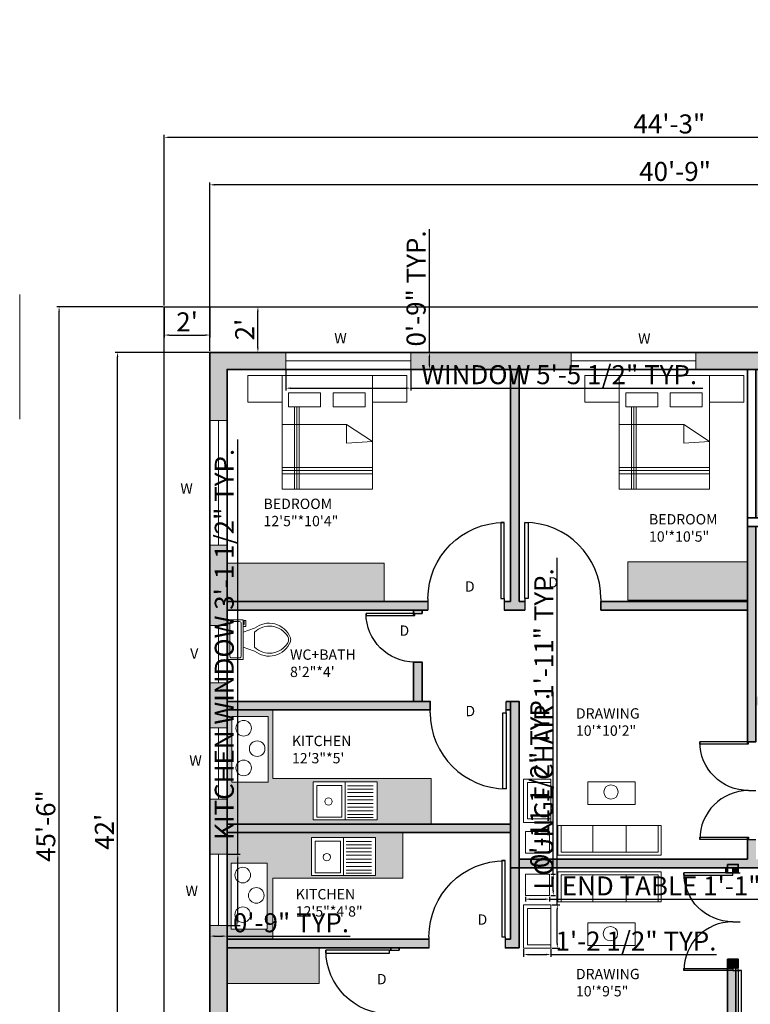
# Model space of a CAD drawing. Units: inches. Extents: x 2048 to 2702, y 2180 to 2964.
# Tile 2 of 3: x 2048 to 2432, y 2447 to 2964. Entities that reach past the tile are written whole.
import ezdxf

# ---------------------------------------------------------------- set-up
doc = ezdxf.new("R2010")
doc.units = ezdxf.units.IN
for name, color, linetype, lineweight in [('A-ANNO-DIMS', 2, 'Continuous', 13), ('A-ANNO-TEXT', 130, 'Continuous', 18), ('A-AREA-IDEN', 130, 'Continuous', 18), ('A-CASE-PATT', 142, 'Continuous', 13), ('A-DOOR', 4, 'Continuous', 25), ('A-EQPM', 142, 'Continuous', 18), ('A-FLOR-FIXT', 142, 'Continuous', 18), ('A-FURN-PATT', 191, 'Continuous', 13), ('A-GLAZ', 4, 'Continuous', 18), ('A-WALL-PATT', 174, 'Continuous', 13), ('bed', 62, 'Continuous', 18), ('C-PROP', 7, 'Continuous', 25), ('kit', 142, 'Continuous', 18), ('sofa', 10, 'Continuous', 18), ('TOI', 210, 'Continuous', 18), ('wall', 174, 'Continuous', 35), ('ward', 191, 'Continuous', 18)]:
    doc.layers.add(name, color=color, linetype=linetype, lineweight=lineweight)
doc.styles.get("Standard").update_dxf_attribs({"font": 'arial.ttf'})
doc.dimstyles.new('ISO-25', dxfattribs={"dimtxt": 10, "dimasz": 2.5, "dimexe": 1.25, "dimexo": 0.625, "dimtad": 1, "dimdec": 0, "dimlunit": 4, "dimtxsty": 'Standard', "dimcen": 2.5, "dimadec": 0, "dimazin": 0, "dimtfac": 1, "dimtdec": 0, "dimtmove": 0, "dimatfit": 3, "dimfxl": 1, "dimarcsym": 0})

# ---------------------------------------------------------------- blocks, each defined once
blk = doc.blocks.new('*U2')
for p, q in [((0, 0), (0, -6)), ((40, 0), (40, -6))]:
    blk.add_line(p, q)
blk.add_lwpolyline([(0, 0), (0, 40), (1.75, 40), (1.75, 0)], close=True)
blk.add_arc((0, 0), 40, 0, 90)
blk = doc.blocks.new('*U4')
for p, q in [((9.5, -6), (9.5, -2)), ((-10, -8.5), (-8, -8.5)), ((-10, -9.5), (-10, -8.5)), ((-7, -9.5), (-10, -9.5)), ((-8, -8.5), (-8, -8)), ((-7, -8), (-7, -9.5)), ((-4, -8), (-6, -14)), ((4, -8), (6, -14)), ((4, -14), (-4, -14))]:
    blk.add_line(p, q)
blk.add_lwpolyline([(10.5, -8), (10.5, 0), (-10.5, 0), (-10.5, -8)], close=True)
for points in [[(-9.5, -2), (-9.5, -6)], [(8.5, -1), (-8.5, -1)], [(-8.5, -7), (8.5, -7)]]:
    blk.add_lwpolyline(points)
for centre, radius, start, end in [((-8.62, -1.88), 0.884, 81.8699, 188.1301), ((8.62, -1.88), 0.884, 351.8699, 98.1301), ((-8.62, -6.12), 0.884, 171.8699, 278.1301), ((8.62, -6.12), 0.884, 261.8699, 8.1301), ((3.52, -21.58), 12.17, 141.4691, 247.9714), ((4.2, -21.82), 11.33, 136.3677, 238.9468), ((-3.52, -21.58), 12.17, 292.0284, 38.5307), ((-4.2, -21.82), 11.33, 301.053, 43.6321), ((0, -27.88), 4, 245.7318, 294.2682), ((0, -29), 4, 254.8605, 285.1395)]:
    blk.add_arc(centre, radius, start, end)
blk = doc.blocks.new('*D7')
at = {"layer": 'A-ANNO-DIMS', "color": 0, "lineweight": -2, "transparency": 16777216}
for p, q in [((2148.03, 2790.14), (2148.03, 2878.84)), ((2637.03, 2790.14), (2637.03, 2878.84)), ((2634.53, 2877.59), (2150.53, 2877.59))]:
    blk.add_line(p, q, dxfattribs=at)
at = {"layer": 'A-ANNO-DIMS', "color": 0, "transparency": 16777216}
for points in [[(2150.53, 2878), (2150.53, 2877.17), (2148.03, 2877.59)], [(2634.53, 2878), (2634.53, 2877.17), (2637.03, 2877.59)]]:
    blk.add_solid(points, dxfattribs=at)
at = {"layer": 'Defpoints', "color": 0, "transparency": 16777216}
for p in [(2148.03, 2877.59), (2148.03, 2789.51), (2637.03, 2789.51)]:
    blk.add_point(p, dxfattribs=at)
at = {"layer": 'A-ANNO-DIMS', "color": 0, "transparency": 16777216, "insert": (2392.53, 2883.32), "char_height": 10, "attachment_point": 5}
blk.add_mtext('40\'-9"', dxfattribs=at)
blk = doc.blocks.new('*D8')
at = {"layer": 'A-ANNO-DIMS', "color": 0, "lineweight": -2, "transparency": 16777216}
for p, q in [((2124.03, 2814.14), (2124.03, 2903.8)), ((2655.03, 2814.14), (2655.03, 2903.8)), ((2126.53, 2902.55), (2652.53, 2902.55))]:
    blk.add_line(p, q, dxfattribs=at)
at = {"layer": 'A-ANNO-DIMS', "color": 0, "transparency": 16777216}
for points in [[(2126.53, 2902.96), (2126.53, 2902.13), (2124.03, 2902.55)], [(2652.53, 2902.96), (2652.53, 2902.13), (2655.03, 2902.55)]]:
    blk.add_solid(points, dxfattribs=at)
at = {"layer": 'Defpoints', "color": 0, "transparency": 16777216}
for p in [(2655.03, 2902.55), (2124.03, 2813.51), (2655.03, 2813.51)]:
    blk.add_point(p, dxfattribs=at)
at = {"layer": 'A-ANNO-DIMS', "color": 0, "transparency": 16777216, "insert": (2389.53, 2908.28), "char_height": 10, "attachment_point": 5}
blk.add_mtext('44\'-3"', dxfattribs=at)
blk = doc.blocks.new('*D9')
at = {"layer": 'A-ANNO-DIMS', "color": 0, "lineweight": -2, "transparency": 16777216}
for p, q in [((2124.03, 2812.89), (2124.03, 2797.35)), ((2148.03, 2812.89), (2148.03, 2797.35)), ((2126.53, 2798.6), (2145.53, 2798.6))]:
    blk.add_line(p, q, dxfattribs=at)
at = {"layer": 'A-ANNO-DIMS', "color": 0, "transparency": 16777216}
for points in [[(2126.53, 2799.01), (2126.53, 2798.18), (2124.03, 2798.6)], [(2145.53, 2799.01), (2145.53, 2798.18), (2148.03, 2798.6)]]:
    blk.add_solid(points, dxfattribs=at)
at = {"layer": 'Defpoints', "color": 0, "transparency": 16777216}
for p in [(2124.03, 2813.51), (2148.03, 2813.51), (2148.03, 2798.6)]:
    blk.add_point(p, dxfattribs=at)
at = {"layer": 'A-ANNO-DIMS', "color": 0, "transparency": 16777216, "insert": (2136.03, 2804.24), "char_height": 10, "attachment_point": 5}
blk.add_mtext("2'", dxfattribs=at)
blk = doc.blocks.new('*D10')
at = {"layer": 'A-ANNO-DIMS', "color": 0, "lineweight": -2, "transparency": 16777216}
for p, q in [((2148.65, 2813.51), (2174.49, 2813.51)), ((2173.24, 2792.01), (2173.24, 2811.01)), ((2148.65, 2789.51), (2174.49, 2789.51))]:
    blk.add_line(p, q, dxfattribs=at)
at = {"layer": 'A-ANNO-DIMS', "color": 0, "transparency": 16777216}
for points in [[(2172.82, 2811.01), (2173.66, 2811.01), (2173.24, 2813.51)], [(2172.82, 2792.01), (2173.66, 2792.01), (2173.24, 2789.51)]]:
    blk.add_solid(points, dxfattribs=at)
at = {"layer": 'Defpoints', "color": 0, "transparency": 16777216}
for p in [(2148.03, 2813.51), (2173.24, 2813.51), (2148.03, 2789.51)]:
    blk.add_point(p, dxfattribs=at)
at = {"layer": 'A-ANNO-DIMS', "color": 0, "transparency": 16777216, "insert": (2167.6, 2801.51), "char_height": 10, "attachment_point": 5, "rotation": 90}
blk.add_mtext("2'", dxfattribs=at)
blk = doc.blocks.new('*D11')
at = {"layer": 'A-ANNO-DIMS', "color": 0, "lineweight": -2, "transparency": 16777216}
for p, q in [((2123.4, 2813.51), (2067.51, 2813.51)), ((2068.76, 2270.01), (2068.76, 2811.01)), ((2123.4, 2267.51), (2067.51, 2267.51))]:
    blk.add_line(p, q, dxfattribs=at)
at = {"layer": 'A-ANNO-DIMS', "color": 0, "transparency": 16777216}
for points in [[(2068.35, 2811.01), (2069.18, 2811.01), (2068.76, 2813.51)], [(2068.35, 2270.01), (2069.18, 2270.01), (2068.76, 2267.51)]]:
    blk.add_solid(points, dxfattribs=at)
at = {"layer": 'Defpoints', "color": 0, "transparency": 16777216}
for p in [(2068.76, 2813.51), (2124.03, 2813.51), (2124.03, 2267.51)]:
    blk.add_point(p, dxfattribs=at)
at = {"layer": 'A-ANNO-DIMS', "color": 0, "transparency": 16777216, "insert": (2063.03, 2540.51), "char_height": 10, "attachment_point": 5, "rotation": 90}
blk.add_mtext('45\'-6"', dxfattribs=at)
blk = doc.blocks.new('*D12')
at = {"layer": 'A-ANNO-DIMS', "color": 0, "lineweight": -2, "transparency": 16777216}
for p, q in [((2147.4, 2789.51), (2098.23, 2789.51)), ((2099.48, 2288.01), (2099.48, 2787.01)), ((2147.4, 2285.51), (2098.23, 2285.51))]:
    blk.add_line(p, q, dxfattribs=at)
at = {"layer": 'A-ANNO-DIMS', "color": 0, "transparency": 16777216}
for points in [[(2099.06, 2787.01), (2099.89, 2787.01), (2099.48, 2789.51)], [(2099.06, 2288.01), (2099.89, 2288.01), (2099.48, 2285.51)]]:
    blk.add_solid(points, dxfattribs=at)
at = {"layer": 'Defpoints', "color": 0, "transparency": 16777216}
for p in [(2099.48, 2789.51), (2148.03, 2789.51), (2148.03, 2285.51)]:
    blk.add_point(p, dxfattribs=at)
at = {"layer": 'A-ANNO-DIMS', "color": 0, "transparency": 16777216, "insert": (2093.83, 2537.51), "char_height": 10, "attachment_point": 5, "rotation": 90}
blk.add_mtext("42'", dxfattribs=at)
blk = doc.blocks.new('BED-DOUBLE-NIGHTSTANDS')
for p, q in [((24.5, 43.17), (24.5, 0)), ((25.71, 43.17), (25.71, 0)), ((26.92, 43.17), (26.92, 0)), ((18.01, 33.96), (51.87, 33.96)), ((51.87, 33.96), (65.5, 24.98)), ((51.87, 24.18), (51.87, 33.96)), ((65.5, 24.98), (51.87, 24.18)), ((18.01, 11.29), (65.5, 11.29)), ((18.01, 9.68), (65.5, 9.68)), ((18.01, 8.07), (65.5, 8.07))]:
    blk.add_line(p, q)
for points in [[(18.01, 59.74), (0, 59.74), (0, 45.7), (18.01, 45.7)], [(18.01, 59.74), (65.5, 59.74), (65.5, 0), (18.01, 0)], [(83.51, 59.74), (65.5, 59.74), (65.5, 45.7), (83.51, 45.7)], [(21.39, 50.51), (38.23, 50.51), (38.23, 43.17), (21.39, 43.17)], [(44.78, 50.51), (61.62, 50.51), (61.62, 43.17), (44.78, 43.17)]]:
    blk.add_lwpolyline(points, close=True)
blk = doc.blocks.new('COOKTOP-3-BURNER')
blk.add_lwpolyline([(0, 0), (34.65, 0), (34.65, 18.99), (0, 18.99)], close=True)
for centre in [(6.24, 12.85), (27.06, 12.85), (16.95, 5.75)]:
    blk.add_circle(centre, 4.1)
blk = doc.blocks.new('SINK-WITH-DRAINER')
for p, q in [((2.08, 18.11), (2.08, 31.52)), ((3.85, 18.11), (3.85, 31.52)), ((5.62, 18.11), (5.62, 31.52)), ((7.59, 18.11), (7.59, 31.52)), ((9.36, 18.11), (9.36, 31.52)), ((11.32, 18.11), (11.32, 31.52)), ((13.22, 18.11), (13.22, 31.52)), ((15.25, 18.11), (15.25, 31.52)), ((17.15, 18.11), (17.15, 31.52)), ((18.67, 18.11), (18.67, 31.52)), ((0, 16.82), (19.98, 16.82))]:
    blk.add_line(p, q)
for points in [[(0, 0), (19.98, 0), (19.98, 33.65), (0, 33.65)], [(1.93, 1.93), (18.53, 1.93), (18.53, 15.13), (1.93, 15.13)]]:
    blk.add_lwpolyline(points, close=True)
blk.add_circle((10.31, 8.05), 1.95)
blk = doc.blocks.new('WINDOW-WIDE')
blk.add_line((0, 4.49), (65.63, 4.49))
blk.add_lwpolyline([(0, 0), (65.63, 0), (65.63, 8.99), (0, 8.99)], close=True)
blk = doc.blocks.new('WINDOW-KITCHEN-NARROW')
blk.add_line((4.5, 0), (4.5, 37.53))
blk.add_lwpolyline([(0, 0), (9, 0), (9, 37.53), (0, 37.53)], close=True)
blk = doc.blocks.new('LOUNGE-CHAIR')
for p, q in [((0, 0), (0, 22.78)), ((0, 22.78), (14.27, 22.78)), ((14.27, 22.78), (14.27, 17.76)), ((14.27, 0), (0, 0)), ((14.27, 1.72), (14.27, 0))]:
    blk.add_line(p, q)
blk.add_lwpolyline([(2, 20.8), (14.27, 20.8), (14.27, 1.72), (2, 1.72)], close=True)
blk = doc.blocks.new('END-TABLE')
blk.add_lwpolyline([(0, 11.28), (12.75, 11.28), (12.75, 0), (0, 0)], close=True)
blk = doc.blocks.new('*D25')
at = {"layer": 'A-ANNO-DIMS', "color": 0, "lineweight": -2, "transparency": 16777216}
for p, q in [((2187.94, 2779.9), (2187.94, 2769.43)), ((2253.56, 2779.9), (2253.56, 2769.43)), ((2190.44, 2770.68), (2251.06, 2770.68)), ((2253.56, 2770.68), (2407.16, 2770.68))]:
    blk.add_line(p, q, dxfattribs=at)
at = {"layer": 'A-ANNO-DIMS', "color": 0, "transparency": 16777216}
for points in [[(2190.44, 2771.09), (2190.44, 2770.26), (2187.94, 2770.68)], [(2251.06, 2771.09), (2251.06, 2770.26), (2253.56, 2770.68)]]:
    blk.add_solid(points, dxfattribs=at)
at = {"layer": 'Defpoints', "color": 0, "transparency": 16777216}
for p in [(2187.94, 2780.52), (2253.56, 2780.52), (2253.56, 2770.68)]:
    blk.add_point(p, dxfattribs=at)
at = {"layer": 'A-ANNO-DIMS', "color": 0, "transparency": 16777216, "insert": (2331.61, 2776.48), "char_height": 10, "attachment_point": 5}
blk.add_mtext('WINDOW 5\'-5 1/2" TYP.', dxfattribs=at)
blk = doc.blocks.new('*D26')
at = {"layer": 'A-ANNO-DIMS', "color": 0, "lineweight": -2, "transparency": 16777216}
for p, q in [((2263.41, 2789.51), (2263.41, 2854.22)), ((2254.19, 2789.51), (2264.66, 2789.51)), ((2263.41, 2783.02), (2263.41, 2787.01)), ((2254.19, 2780.52), (2264.66, 2780.52))]:
    blk.add_line(p, q, dxfattribs=at)
at = {"layer": 'A-ANNO-DIMS', "color": 0, "transparency": 16777216}
for points in [[(2262.99, 2787.01), (2263.83, 2787.01), (2263.41, 2789.51)], [(2262.99, 2783.02), (2263.83, 2783.02), (2263.41, 2780.52)]]:
    blk.add_solid(points, dxfattribs=at)
at = {"layer": 'Defpoints', "color": 0, "transparency": 16777216}
for p in [(2253.56, 2789.51), (2263.41, 2789.51), (2253.56, 2780.52)]:
    blk.add_point(p, dxfattribs=at)
at = {"layer": 'A-ANNO-DIMS', "color": 0, "transparency": 16777216, "insert": (2257.68, 2823.11), "char_height": 10, "attachment_point": 5, "rotation": 90}
blk.add_mtext('0\'-9" TYP.', dxfattribs=at)
blk = doc.blocks.new('*D27')
at = {"layer": 'A-ANNO-DIMS', "color": 0, "lineweight": -2, "transparency": 16777216}
for p, q in [((2462.17, 2739.8), (2462.17, 2964.38)), ((2457.74, 2739.8), (2463.42, 2739.8)), ((2462.17, 2708.66), (2462.17, 2737.3)), ((2457.74, 2706.16), (2463.42, 2706.16))]:
    blk.add_line(p, q, dxfattribs=at)
at = {"layer": 'A-ANNO-DIMS', "color": 0, "transparency": 16777216}
for points in [[(2461.75, 2737.3), (2462.58, 2737.3), (2462.17, 2739.8)], [(2461.75, 2708.66), (2462.58, 2708.66), (2462.17, 2706.16)]]:
    blk.add_solid(points, dxfattribs=at)
at = {"layer": 'Defpoints', "color": 0, "transparency": 16777216}
for p in [(2457.12, 2739.8), (2462.17, 2739.8), (2457.12, 2706.16)]:
    blk.add_point(p, dxfattribs=at)
at = {"layer": 'A-ANNO-DIMS', "color": 0, "transparency": 16777216, "insert": (2456.37, 2853.34), "char_height": 10, "attachment_point": 5, "rotation": 90}
blk.add_mtext('SINK AND DRAINER 2\'-9 1/2" TYP.', dxfattribs=at)
blk = doc.blocks.new('*D33')
at = {"layer": 'A-ANNO-DIMS', "color": 0, "lineweight": -2, "transparency": 16777216}
for p, q in [((2162.66, 2525.8), (2162.66, 2743.74)), ((2157.65, 2525.8), (2163.91, 2525.8)), ((2162.66, 2490.77), (2162.66, 2523.3)), ((2157.65, 2488.27), (2163.91, 2488.27))]:
    blk.add_line(p, q, dxfattribs=at)
at = {"layer": 'A-ANNO-DIMS', "color": 0, "transparency": 16777216}
for points in [[(2162.24, 2523.3), (2163.07, 2523.3), (2162.66, 2525.8)], [(2162.24, 2490.77), (2163.07, 2490.77), (2162.66, 2488.27)]]:
    blk.add_solid(points, dxfattribs=at)
at = {"layer": 'Defpoints', "color": 0, "transparency": 16777216}
for p in [(2157.03, 2525.8), (2162.66, 2525.8), (2157.03, 2488.27)]:
    blk.add_point(p, dxfattribs=at)
at = {"layer": 'A-ANNO-DIMS', "color": 0, "transparency": 16777216, "insert": (2156.85, 2636.02), "char_height": 10, "attachment_point": 5, "rotation": 90}
blk.add_mtext('KITCHEN WINDOW 3\'-1 1/2" TYP.', dxfattribs=at)
blk = doc.blocks.new('*D34')
at = {"layer": 'A-ANNO-DIMS', "color": 0, "lineweight": -2, "transparency": 16777216}
for p, q in [((2148.03, 2487.64), (2148.03, 2481.39)), ((2157.03, 2487.64), (2157.03, 2481.39)), ((2150.53, 2482.64), (2154.53, 2482.64)), ((2157.03, 2482.64), (2221.73, 2482.64))]:
    blk.add_line(p, q, dxfattribs=at)
at = {"layer": 'A-ANNO-DIMS', "color": 0, "transparency": 16777216}
for points in [[(2150.53, 2483.05), (2150.53, 2482.22), (2148.03, 2482.64)], [(2154.53, 2483.05), (2154.53, 2482.22), (2157.03, 2482.64)]]:
    blk.add_solid(points, dxfattribs=at)
at = {"layer": 'Defpoints', "color": 0, "transparency": 16777216}
for p in [(2148.03, 2488.27), (2157.03, 2488.27), (2157.03, 2482.64)]:
    blk.add_point(p, dxfattribs=at)
at = {"layer": 'A-ANNO-DIMS', "color": 0, "transparency": 16777216, "insert": (2190.63, 2488.37), "char_height": 10, "attachment_point": 5}
blk.add_mtext('0\'-9" TYP.', dxfattribs=at)
blk = doc.blocks.new('*D35')
at = {"layer": 'A-ANNO-DIMS', "color": 0, "lineweight": -2, "transparency": 16777216}
for p, q in [((2330.62, 2499.16), (2330.62, 2681.42)), ((2327.82, 2499.16), (2331.87, 2499.16)), ((2330.62, 2478.88), (2330.62, 2496.66)), ((2327.82, 2476.38), (2331.87, 2476.38))]:
    blk.add_line(p, q, dxfattribs=at)
at = {"layer": 'A-ANNO-DIMS', "color": 0, "transparency": 16777216}
for points in [[(2330.2, 2496.66), (2331.03, 2496.66), (2330.62, 2499.16)], [(2330.2, 2478.88), (2331.03, 2478.88), (2330.62, 2476.38)]]:
    blk.add_solid(points, dxfattribs=at)
at = {"layer": 'Defpoints', "color": 0, "transparency": 16777216}
for p in [(2327.2, 2499.16), (2330.62, 2499.16), (2327.2, 2476.38)]:
    blk.add_point(p, dxfattribs=at)
at = {"layer": 'A-ANNO-DIMS', "color": 0, "transparency": 16777216, "insert": (2324.82, 2591.54), "char_height": 10, "attachment_point": 5, "rotation": 90}
blk.add_mtext('LOUNGE CHAIR 1\'-11" TYP.', dxfattribs=at)
blk = doc.blocks.new('*D36')
at = {"layer": 'A-ANNO-DIMS', "color": 0, "lineweight": -2, "transparency": 16777216}
for p, q in [((2312.93, 2475.76), (2312.93, 2471.72)), ((2327.2, 2475.76), (2327.2, 2471.72)), ((2315.43, 2472.97), (2324.7, 2472.97)), ((2327.2, 2472.97), (2414.26, 2472.97))]:
    blk.add_line(p, q, dxfattribs=at)
at = {"layer": 'A-ANNO-DIMS', "color": 0, "transparency": 16777216}
for points in [[(2315.43, 2473.38), (2315.43, 2472.55), (2312.93, 2472.97)], [(2324.7, 2473.38), (2324.7, 2472.55), (2327.2, 2472.97)]]:
    blk.add_solid(points, dxfattribs=at)
at = {"layer": 'Defpoints', "color": 0, "transparency": 16777216}
for p in [(2312.93, 2476.38), (2327.2, 2476.38), (2327.2, 2472.97)]:
    blk.add_point(p, dxfattribs=at)
at = {"layer": 'A-ANNO-DIMS', "color": 0, "transparency": 16777216, "insert": (2371.98, 2478.76), "char_height": 10, "attachment_point": 5}
blk.add_mtext('1\'-2 1/2" TYP.', dxfattribs=at)
blk = doc.blocks.new('*D37')
at = {"layer": 'A-ANNO-DIMS', "color": 0, "lineweight": -2, "transparency": 16777216}
for p, q in [((2313.82, 2503.37), (2313.82, 2500.83)), ((2316.32, 2502.08), (2324.08, 2502.08)), ((2326.58, 2503.37), (2326.58, 2500.83)), ((2326.58, 2502.08), (2472.27, 2502.08))]:
    blk.add_line(p, q, dxfattribs=at)
at = {"layer": 'A-ANNO-DIMS', "color": 0, "transparency": 16777216}
for points in [[(2316.32, 2502.5), (2316.32, 2501.66), (2313.82, 2502.08)], [(2324.08, 2502.5), (2324.08, 2501.66), (2326.58, 2502.08)]]:
    blk.add_solid(points, dxfattribs=at)
at = {"layer": 'Defpoints', "color": 0, "transparency": 16777216}
for p in [(2313.82, 2503.99), (2326.58, 2503.99), (2326.58, 2502.08)]:
    blk.add_point(p, dxfattribs=at)
at = {"layer": 'A-ANNO-DIMS', "color": 0, "transparency": 16777216, "insert": (2400.67, 2507.73), "char_height": 10, "attachment_point": 5}
blk.add_mtext('END TABLE 1\'-1" TYP.', dxfattribs=at)
blk = doc.blocks.new('*D38')
at = {"layer": 'A-ANNO-DIMS', "color": 0, "lineweight": -2, "transparency": 16777216}
for p, q in [((2328.49, 2515.28), (2328.49, 2611.05)), ((2327.2, 2515.28), (2329.74, 2515.28)), ((2328.49, 2506.49), (2328.49, 2512.78)), ((2327.2, 2503.99), (2329.74, 2503.99))]:
    blk.add_line(p, q, dxfattribs=at)
at = {"layer": 'A-ANNO-DIMS', "color": 0, "transparency": 16777216}
for points in [[(2328.07, 2512.78), (2328.91, 2512.78), (2328.49, 2515.28)], [(2328.07, 2506.49), (2328.91, 2506.49), (2328.49, 2503.99)]]:
    blk.add_solid(points, dxfattribs=at)
at = {"layer": 'Defpoints', "color": 0, "transparency": 16777216}
for p in [(2326.58, 2515.28), (2328.49, 2515.28), (2326.58, 2503.99)]:
    blk.add_point(p, dxfattribs=at)
at = {"layer": 'A-ANNO-DIMS', "color": 0, "transparency": 16777216, "insert": (2322.7, 2564.42), "char_height": 10, "attachment_point": 5, "rotation": 90}
blk.add_mtext('0\'-11 1/2" TYP.', dxfattribs=at)

msp = doc.modelspace()

# ---------------------------------------------------------------- hatches: boundary and pattern name
at = {"layer": 'A-CASE-PATT'}
h = msp.add_hatch(color=256, dxfattribs=at)
h.dxf.hatch_style = 1
h.paths.add_polyline_path([(2264.28, 2565.56), (2181.03, 2565.56), (2181.03, 2601.56), (2157.03, 2601.56), (2157.03, 2541.56), (2264.28, 2541.56)])
h.paths.add_polyline_path([(2178.6, 2563.49), (2159.62, 2563.49), (2159.62, 2598.14), (2178.6, 2598.14)], flags=16)
h.paths.add_polyline_path([(2161.65, 2571.08, -1), (2169.85, 2571.08, -1)], flags=0)
h.paths.add_polyline_path([(2202.29, 2563.69), (2235.94, 2563.69), (2235.94, 2543.71), (2202.29, 2543.71)], flags=16)
h.paths.add_polyline_path([(2204.22, 2561.75), (2217.42, 2561.75), (2217.42, 2545.16), (2204.22, 2545.16)], flags=0)
h.paths.add_polyline_path([(2168.75, 2581.19, -1), (2176.95, 2581.19, -1)], flags=0)
h.paths.add_polyline_path([(2212.29, 2553.38, -1), (2208.39, 2553.38, -1)], flags=0)
h.paths.add_polyline_path([(2161.65, 2591.9, -1), (2169.85, 2591.9, -1)], flags=0)
h.paths.add_polyline_path([(2249.43, 2537.06), (2157.03, 2537.06), (2157.03, 2481.06), (2181.03, 2481.06), (2181.03, 2513.06), (2249.43, 2513.06)])
h.paths.add_polyline_path([(2178.15, 2520.97), (2178.15, 2486.32), (2159.16, 2486.32), (2159.16, 2520.97)], flags=16)
h.paths.add_polyline_path([(2201.45, 2534.49), (2235.1, 2534.49), (2235.1, 2514.51), (2201.45, 2514.51)], flags=16)
h.paths.add_polyline_path([(2203.38, 2532.56), (2216.58, 2532.56), (2216.58, 2515.96), (2203.38, 2515.96)], flags=0)
h.paths.add_polyline_path([(2169.4, 2514.73, -1), (2161.2, 2514.73, -1)], flags=0)
h.paths.add_polyline_path([(2176.5, 2504.02, -1), (2168.3, 2504.02, -1)], flags=0)
h.paths.add_polyline_path([(2211.45, 2524.18, -1), (2207.55, 2524.18, -1)], flags=0)
h.paths.add_polyline_path([(2169.4, 2493.91, -1), (2161.2, 2493.91, -1)], flags=0)
h.paths.add_polyline_path([(2628.03, 2372.19), (2627.36, 2372.19), (2627.36, 2424), (2604.03, 2424), (2604.03, 2365.01), (2568.03, 2365.01), (2568.03, 2341.01), (2628.03, 2341.01)])
h.paths.add_polyline_path([(2606.7, 2374.82), (2606.7, 2409.47), (2625.69, 2409.47), (2625.69, 2374.82)], flags=16)
h.paths.add_polyline_path([(2604.57, 2362.79), (2604.57, 2342.81), (2570.92, 2342.81), (2570.92, 2362.79)], flags=16)
h.paths.add_polyline_path([(2615.46, 2382.4, -1), (2623.66, 2382.4, -1)], flags=0)
h.paths.add_polyline_path([(2608.36, 2392.51, -1), (2616.56, 2392.51, -1)], flags=0)
h.paths.add_polyline_path([(2586.06, 2360.86), (2586.06, 2344.26), (2572.85, 2344.26), (2572.85, 2360.86)], flags=0)
h.paths.add_polyline_path([(2615.46, 2403.23, -1), (2623.66, 2403.23, -1)], flags=0)
h.paths.add_polyline_path([(2580.92, 2352.48, -1), (2577.03, 2352.48, -1)], flags=0)
h.paths.add_polyline_path([(2517.03, 2780.51), (2435.03, 2780.51), (2435.03, 2702.51), (2459.03, 2702.51), (2459.03, 2756.51), (2517.03, 2756.51)])
h.paths.add_polyline_path([(2468.7, 2777.39), (2503.35, 2777.39), (2503.35, 2758.41), (2468.7, 2758.41)], flags=16)
h.paths.add_polyline_path([(2470.84, 2771.26, -1), (2479.04, 2771.26, -1)], flags=0)
h.paths.add_polyline_path([(2457.12, 2739.8), (2457.12, 2706.16), (2437.14, 2706.16), (2437.14, 2739.8)], flags=16)
h.paths.add_polyline_path([(2489.75, 2764.16, -1), (2481.55, 2764.16, -1)], flags=0)
h.paths.add_polyline_path([(2491.66, 2771.26, -1), (2499.86, 2771.26, -1)], flags=0)
h.paths.add_polyline_path([(2455.67, 2721.29), (2455.67, 2708.09), (2439.07, 2708.09), (2439.07, 2721.29)], flags=0)
h.paths.add_polyline_path([(2449.4, 2714.21, -1), (2445.51, 2714.21, -1)], flags=0)
at = {"layer": 'A-FURN-PATT'}
h = msp.add_hatch(color=256, dxfattribs=at)
h.dxf.hatch_style = 1
h.paths.add_polyline_path([(2239.55, 2678.76), (2157.03, 2678.76), (2157.03, 2658.56), (2239.55, 2658.56)])
h.paths.add_polyline_path([(2430.53, 2679.37), (2367.61, 2679.37), (2367.61, 2659.17), (2430.53, 2659.17)])
h.paths.add_polyline_path([(2628.03, 2681.82), (2565.11, 2681.82), (2565.11, 2661.62), (2628.03, 2661.62)])
h = msp.add_hatch(color=256, dxfattribs=at)
h.dxf.hatch_style = 1
h.paths.add_polyline_path([(2205.4, 2476.56), (2157.03, 2476.56), (2157.03, 2457.66), (2205.4, 2457.66)])
h.paths.add_polyline_path([(2420.03, 2414.51), (2352.49, 2414.51), (2352.49, 2393.19), (2420.03, 2393.19)])
at = {"layer": 'A-WALL-PATT'}
h = msp.add_hatch(color=256, dxfattribs=at)
h.dxf.hatch_style = 1
h.paths.add_polyline_path([(2187.94, 2789.51), (2148.03, 2789.51), (2148.03, 2753.7), (2157.03, 2753.7), (2157.03, 2780.51), (2187.94, 2780.52)])
h.paths.add_polyline_path([(2337.86, 2789.51), (2253.56, 2789.51), (2253.56, 2780.55), (2306.03, 2780.56), (2310.53, 2780.56), (2310.53, 2780.56), (2337.86, 2780.56)])
h.paths.add_polyline_path([(2442.77, 2789.51), (2403.49, 2789.51), (2403.49, 2780.56), (2430.53, 2780.56), (2442.77, 2780.56)])
h.paths.add_polyline_path([(2157.03, 2678.76), (2157.03, 2688.07), (2148.03, 2688.07), (2148.03, 2645.92), (2157.03, 2645.92), (2157.03, 2658.56), (2157.03, 2658.56)])
h = msp.add_hatch(color=256, dxfattribs=at)
h.dxf.hatch_style = 1
h.paths.add_polyline_path([(2310.53, 2780.51), (2306.03, 2780.51), (2306.03, 2658.56), (2302.65, 2658.56), (2302.65, 2654.06), (2310.53, 2654.06), (2313.53, 2654.06), (2313.53, 2658.56), (2310.53, 2658.56)])
h.paths.add_polyline_path([(2262.65, 2658.56), (2157.03, 2658.56), (2157.03, 2654.06), (2255.03, 2654.06), (2262.65, 2654.06)])
h.paths.add_polyline_path([(2521.53, 2780.51), (2517.03, 2780.51), (2517.03, 2702.51), (2512.47, 2702.51), (2512.47, 2698.01), (2517.03, 2698.01), (2517.03, 2696.35), (2521.53, 2696.35), (2521.53, 2698.01)])
h.paths.add_polyline_path([(2628.03, 2608.51), (2521.53, 2608.51), (2521.53, 2610.77), (2521, 2610.77), (2517.03, 2610.77), (2517.03, 2608.51), (2487.03, 2608.51), (2478.14, 2608.51), (2478.14, 2604.01), (2487.03, 2604.01), (2592.01, 2604.01), (2628.03, 2604.01)])
h = msp.add_hatch(color=256, dxfattribs=at)
h.dxf.hatch_style = 1
h.paths.add_polyline_path([(2300.03, 2293.61), (2295.53, 2293.61), (2295.53, 2290.01), (2300.03, 2290.01)], flags=17)
h.paths.add_polyline_path([(2637.03, 2290.01), (2632.53, 2290.01), (2568.03, 2290.01), (2424.53, 2290.01), (2424.53, 2289.93), (2420.03, 2290.01), (2295.53, 2290.01), (2152.53, 2290.01), (2152.53, 2336.51), (2148.03, 2336.51), (2148.03, 2285.51), (2637.03, 2285.51)])
h.paths.add_polyline_path([(2424.53, 2465.93), (2420.03, 2466.01), (2420.03, 2290.01), (2424.53, 2289.93)])
h.paths.add_polyline_path([(2420.03, 2419.01), (2343.92, 2419.01), (2343.92, 2414.51), (2420.03, 2414.51)])
h.paths.add_polyline_path([(2637.03, 2522.1), (2628.03, 2522.1), (2628.03, 2508.22), (2637.03, 2508.22)])
h.paths.add_polyline_path([(2263.8, 2606.06), (2157.03, 2606.06), (2157.03, 2601.56), (2263.8, 2601.56)])
h.paths.add_polyline_path([(2259.53, 2626.68), (2255.69, 2626.68, -0.004462), (2255.23, 2626.68), (2255.03, 2626.68), (2255.03, 2606.07), (2259.53, 2606.06)])
h.paths.add_polyline_path([(2259.53, 2654.06), (2255.03, 2654.06), (2255.03, 2652.27), (2255.69, 2652.27), (2259.53, 2652.27)])
h.paths.add_polyline_path([(2310.53, 2606.06), (2306.03, 2606.06), (2306.03, 2518.51), (2310.53, 2518.51)])
h.paths.add_polyline_path([(2306.03, 2606.06), (2303.8, 2606.06), (2303.8, 2601.56), (2306.03, 2601.56)])
h.paths.add_polyline_path([(2306.03, 2541.56), (2157.03, 2541.56), (2157.03, 2537.06), (2306.03, 2537.06)])
h.paths.add_polyline_path([(2435.03, 2698.01), (2430.53, 2698.01), (2430.53, 2658.56), (2430.53, 2658.56), (2430.53, 2654.06), (2430.53, 2584.82), (2435.03, 2584.82)])
h.paths.add_polyline_path([(2430.53, 2658.56), (2353.53, 2658.56), (2353.53, 2654.06), (2430.53, 2654.06)])
h.paths.add_polyline_path([(2438.14, 2608.51), (2435.03, 2608.51), (2435.03, 2604.01), (2438.14, 2604.01)])
h = msp.add_hatch(color=256, dxfattribs=at)
h.dxf.hatch_style = 1
h.paths.add_polyline_path([(2157.03, 2615.7), (2148.03, 2615.7), (2148.03, 2592.16), (2157.03, 2592.16), (2157.03, 2601.56)])
h = msp.add_hatch(color=256, dxfattribs=at)
h.dxf.hatch_style = 1
h.paths.add_polyline_path([(2157.03, 2554.63), (2148.03, 2554.63), (2148.03, 2525.8), (2157.03, 2525.8)])
h.paths.add_polyline_path([(2157.03, 2488.27), (2148.03, 2488.27), (2148.03, 2440.26), (2157.03, 2440.26)])
h.paths.add_polyline_path([(2168.96, 2345.51), (2157.03, 2345.51), (2157.03, 2374.63), (2148.03, 2374.63), (2148.03, 2336.51), (2152.53, 2336.51), (2168.96, 2336.51)])
h.paths.add_polyline_path([(2257.35, 2345.51), (2247.53, 2345.51), (2247.53, 2429.51), (2247.53, 2441.68), (2243.03, 2441.68), (2243.03, 2434.01), (2243.03, 2345.51), (2226.28, 2345.51), (2226.28, 2336.51), (2257.35, 2336.51)])
h.paths.add_polyline_path([(2300.03, 2414.51), (2303.92, 2414.51), (2303.92, 2419.01), (2300.03, 2419.01), (2300.03, 2434.01), (2277.86, 2434.01), (2277.86, 2429.51), (2295.53, 2429.51), (2295.53, 2409.26), (2295.53, 2345.51), (2283.92, 2345.51), (2283.92, 2336.51), (2295.53, 2336.51), (2295.53, 2327.38), (2300.03, 2327.38)])
h.paths.add_polyline_path([(2637.03, 2481.91), (2628.03, 2481.91), (2628.03, 2470.51), (2521.21, 2470.51), (2521.21, 2466.01), (2563.53, 2466.01), (2563.53, 2460.5), (2568.03, 2460.5), (2568.03, 2466.01), (2628.03, 2466.01), (2628.03, 2437.82), (2636.35, 2437.82), (2636.35, 2372.19), (2628.03, 2372.19), (2628.03, 2341.01), (2568.03, 2341.01), (2568.03, 2365.01), (2568.03, 2420.5), (2563.53, 2420.5), (2563.53, 2341.01), (2563.53, 2325.13), (2568.03, 2325.13), (2568.03, 2336.51), (2632.53, 2336.51), (2632.53, 2290.01), (2637.03, 2290.01)])
h.paths.add_polyline_path([(2263.16, 2481.06), (2162.03, 2481.06), (2157.03, 2481.06), (2157.03, 2476.56), (2205.4, 2476.56), (2263.16, 2476.56)])
h.paths.add_polyline_path([(2435.03, 2533.49), (2431.18, 2533.49), (2430.53, 2533.49), (2430.53, 2523.01), (2310.53, 2523.01), (2310.53, 2518.51), (2430.53, 2518.51), (2456.56, 2518.51), (2481.53, 2518.51), (2481.53, 2470.51), (2465.77, 2470.51), (2465.77, 2466.01), (2489.41, 2466.01), (2489.41, 2470.51), (2486.03, 2470.51), (2486.03, 2518.51), (2628.03, 2518.51), (2628.03, 2523.01), (2435.03, 2523.01)])
h.paths.add_polyline_path([(2310.53, 2518.51), (2306.03, 2518.51), (2306.03, 2481.06), (2303.16, 2481.06), (2303.16, 2476.56), (2310.53, 2476.56)])
h = msp.add_hatch(dxfattribs=at)
h.set_pattern_fill('ANGLE', color=256)
h.set_pattern_definition([(0, (0, 0), (0, 6.985), [5.08, -1.905]), (90, (0, 0), (-6.985, 4e-16), [5.08, -1.905])])
h.paths.add_polyline_path([(2422.33, 2518.51), (2420.03, 2518.51), (2419.18, 2518.51), (2419.24, 2515.85), (2422.45, 2515.85)])
h = msp.add_hatch(color=256, dxfattribs=at)
h.dxf.hatch_style = 1
h.paths.add_polyline_path([(2425.77, 2518.51), (2422.33, 2518.51), (2422.45, 2515.86), (2425.77, 2515.86)])
h = msp.add_hatch(color=256, dxfattribs=at)
h.dxf.hatch_style = 1
h.paths.add_polyline_path([(2425.77, 2470.51), (2420.03, 2470.51), (2420.03, 2466.01), (2424.53, 2465.93), (2424.53, 2466.01), (2425.77, 2466.01)])

# ---------------------------------------------------------------- linework, layer by layer
at = {"layer": 'A-GLAZ'}
for p, q in [((2048.03, 2819.97), (2048.03, 2754.34)), ((2152.53, 2615.7), (2152.53, 2645.92))]:
    msp.add_line(p, q, dxfattribs=at)
msp.add_lwpolyline([(2148.03, 2645.92), (2157.03, 2645.92), (2157.03, 2615.7), (2148.03, 2615.7)], close=True, dxfattribs=at)
at = {"layer": 'C-PROP'}
for p, q in [((2124.03, 2813.51), (2655.03, 2813.51)), ((2124.03, 2267.51), (2124.03, 2813.51))]:
    msp.add_line(p, q, dxfattribs=at)
at = {"layer": 'kit'}
for p, q in [((2157.03, 2601.56), (2181.03, 2601.56)), ((2181.03, 2601.56), (2181.03, 2565.56)), ((2264.28, 2565.56), (2181.03, 2565.56)), ((2264.28, 2541.56), (2264.28, 2565.56)), ((2242.16, 2537.06), (2244.75, 2537.06)), ((2249.43, 2537.06), (2249.43, 2513.06)), ((2181.03, 2481.06), (2181.03, 2513.06)), ((2249.43, 2513.06), (2181.03, 2513.06)), ((2157.03, 2481.06), (2181.03, 2481.06))]:
    msp.add_line(p, q, dxfattribs=at)
at = {"layer": 'sofa'}
for p, q in [((2332.69, 2540.82), (2330.81, 2540.82)), ((2330.81, 2540.82), (2330.81, 2525.13)), ((2349.3, 2526.72), (2349.3, 2540.82)), ((2366.84, 2526.72), (2366.84, 2540.82)), ((2385.19, 2540.82), (2381.14, 2540.82)), ((2385.19, 2525.13), (2385.19, 2540.82)), ((2330.81, 2525.13), (2385.19, 2525.13)), ((2330.81, 2500.73), (2330.81, 2516.42)), ((2330.81, 2516.42), (2385.19, 2516.42)), ((2385.19, 2516.42), (2385.19, 2500.73)), ((2349.3, 2514.84), (2349.3, 2500.73)), ((2366.84, 2514.84), (2366.84, 2500.73)), ((2332.69, 2500.73), (2330.81, 2500.73)), ((2383.68, 2500.73), (2385.19, 2500.73))]:
    msp.add_line(p, q, dxfattribs=at)
for points in [[(2346.75, 2551.85), (2371.48, 2551.85), (2371.48, 2563.76), (2346.75, 2563.76)], [(2332.69, 2540.82), (2383.68, 2540.82), (2383.68, 2526.72), (2332.69, 2526.72)], [(2332.69, 2500.73), (2383.68, 2500.73), (2383.68, 2514.84), (2332.69, 2514.84)], [(2346.75, 2489.71), (2371.48, 2489.71), (2371.48, 2477.79), (2346.75, 2477.79)]]:
    msp.add_lwpolyline(points, close=True, dxfattribs=at)
for centre in [(2358.84, 2558.4), (2358.53, 2483.93)]:
    msp.add_circle(centre, 3.8, dxfattribs=at)
at = {"layer": 'wall'}
for p, q in [((2157.03, 2780.51), (2306.03, 2780.56)), ((2306.03, 2780.56), (2306.03, 2658.56)), ((2310.53, 2780.56), (2310.53, 2658.56)), ((2310.53, 2780.56), (2430.53, 2780.56)), ((2310.53, 2780.51), (2430.53, 2780.51)), ((2310.53, 2780.51), (2322.53, 2780.51)), ((2430.53, 2780.56), (2430.53, 2658.56)), ((2262.65, 2658.56), (2157.03, 2658.56)), ((2306.03, 2658.56), (2302.65, 2658.56)), ((2310.53, 2658.56), (2313.53, 2658.56)), ((2353.53, 2658.56), (2430.53, 2658.56)), ((2157.03, 2654.06), (2255.03, 2654.06)), ((2262.65, 2654.06), (2157.03, 2654.06)), ((2255.03, 2654.06), (2255.03, 2651.15)), ((2259.53, 2654.06), (2259.53, 2652.27)), ((2310.53, 2654.06), (2302.65, 2654.06)), ((2310.53, 2654.06), (2313.53, 2654.06)), ((2353.53, 2654.06), (2430.53, 2654.06)), ((2430.53, 2654.06), (2430.53, 2583.7)), ((2430.53, 2583.7), (2430.53, 2645.01)), ((2255.03, 2626.68), (2255.03, 2606.06)), ((2259.53, 2626.68), (2259.53, 2606.06)), ((2255.03, 2606.06), (2157.03, 2606.06)), ((2255.03, 2606.06), (2238.1, 2606.06)), ((2263.8, 2606.06), (2259.53, 2606.06)), ((2310.53, 2606.06), (2303.8, 2606.06)), ((2310.53, 2537.06), (2310.53, 2606.06)), ((2259.53, 2601.56), (2157.03, 2601.56)), ((2157.03, 2601.56), (2157.03, 2541.56)), ((2263.8, 2601.56), (2238.1, 2601.56)), ((2306.03, 2601.56), (2303.8, 2601.56)), ((2306.03, 2541.56), (2306.03, 2601.56)), ((2430.53, 2559.15), (2430.53, 2559.16)), ((2157.03, 2541.56), (2306.03, 2541.56)), ((2157.03, 2537.06), (2243.03, 2537.06)), ((2243.46, 2537.06), (2263.26, 2537.06)), ((2247.53, 2537.06), (2306.03, 2537.06)), ((2306.03, 2518.51), (2306.03, 2537.06)), ((2306.03, 2537.06), (2306.03, 2481.06)), ((2310.53, 2537.06), (2310.53, 2523.01)), ((2310.53, 2537.06), (2310.53, 2476.56)), ((2430.53, 2523.01), (2430.53, 2534.61)), ((2310.53, 2523.01), (2430.53, 2523.01)), ((2430.53, 2523.01), (2310.53, 2523.01)), ((2430.53, 2518.51), (2306.03, 2518.51)), ((2419.24, 2515.85), (2419.18, 2518.51)), ((2422.45, 2515.85), (2419.24, 2515.85)), ((2420.03, 2518.51), (2422.33, 2518.51)), ((2422.45, 2515.86), (2422.45, 2515.85)), ((2428.23, 2518.51), (2456.56, 2518.51)), ((2162.03, 2481.06), (2157.03, 2481.06)), ((2263.06, 2481.06), (2162.03, 2481.06)), ((2306.03, 2481.06), (2303.06, 2481.06)), ((2162.03, 2476.56), (2157.03, 2476.56)), ((2263.16, 2476.56), (2162.03, 2476.56)), ((2243.03, 2475.2), (2243.03, 2476.56)), ((2247.53, 2475.2), (2247.53, 2476.56)), ((2310.53, 2476.56), (2303.16, 2476.56)), ((2420.03, 2419.01), (2420.03, 2470.51)), ((2425.77, 2470.51), (2420.03, 2470.51)), ((2424.53, 2294.51), (2424.53, 2466.01)), ((2425.77, 2466.01), (2424.53, 2466.01))]:
    msp.add_line(p, q, dxfattribs=at)
for points in [[(2148.03, 2285.51), (2637.03, 2285.51), (2637.03, 2789.51), (2148.03, 2789.51)], [(2430.53, 2780.51), (2435.03, 2780.51), (2435.03, 2702.51), (2430.53, 2702.51)], [(2472.47, 2698.01), (2430.53, 2698.01), (2430.53, 2702.51), (2472.47, 2702.51)], [(2430.53, 2698.01), (2435.03, 2698.01), (2435.03, 2584.82), (2430.53, 2584.82)], [(2353.53, 2658.56), (2430.53, 2658.56), (2430.53, 2654.06), (2353.53, 2654.06)], [(2255.03, 2626.68), (2259.53, 2626.68), (2259.53, 2606.06), (2255.03, 2606.07)], [(2157.03, 2606.06), (2263.8, 2606.06), (2263.8, 2601.56), (2157.03, 2601.56)], [(2306.03, 2518.51), (2310.53, 2518.51), (2310.53, 2606.06), (2306.03, 2606.06)], [(2157.03, 2541.56), (2306.03, 2541.56), (2306.03, 2537.06), (2157.03, 2537.06)], [(2420.03, 2520.36), (2425.77, 2520.36), (2425.77, 2515.86), (2420.03, 2515.86)], [(2420.03, 2470.51), (2425.77, 2470.51), (2425.77, 2466.01), (2420.03, 2466.01)], [(2420.03, 2290.01), (2424.53, 2289.93), (2424.53, 2465.93), (2420.03, 2466.01)]]:
    msp.add_lwpolyline(points, close=True, dxfattribs=at)
msp.add_lwpolyline([(2628.03, 2661.01), (2628.03, 2780.51), (2157.03, 2780.51), (2157.03, 2345.51)], dxfattribs=at)
at = {"layer": 'ward'}
for points in [[(2157.03, 2658.56), (2239.55, 2658.56), (2239.55, 2678.76), (2157.03, 2678.76)], [(2157.03, 2476.56), (2205.4, 2476.56), (2205.4, 2457.66), (2157.03, 2457.66)]]:
    msp.add_lwpolyline(points, close=True, dxfattribs=at)
msp.add_lwpolyline([(2367.61, 2659.17), (2430.53, 2659.17), (2430.53, 2679.37), (2367.61, 2679.37), (2367.61, 2659.17)], dxfattribs=at)

# ---------------------------------------------------------------- block references
at = {"layer": 'A-DOOR', "xscale": -1}
for p in [(2302.65, 2660.06), (2303.16, 2482.33)]:
    msp.add_blockref('*U2', p, dxfattribs=at)
at = {"layer": 'A-DOOR'}
msp.add_blockref('*U2', (2313.53, 2660.06), dxfattribs=at)
at = {"layer": 'A-DOOR', "rotation": 90}
for p, xscale, yscale, zscale in [((2255.69, 2652.27), -0.6398202342524917, 0.6398202342524917, 0.6398202342524917), ((2431.18, 2584.82), -0.6417118160907794, 0.6417118160907794, 0.6417118160907794), ((2431.18, 2533.49), 0.6417118160907794, 0.6417118160907794, 0.6417118160907794), ((2422.8, 2515.85), -0.6417118160907794, 0.6417118160907794, 0.6417118160907794), ((2422.8, 2464.51), 0.6417118160907794, 0.6417118160907794, 0.6417118160907794), ((2242.5, 2475.2), -0.8377984646543621, 0.8377984646543621, 0.8377984646543621)]:
    msp.add_blockref('*U2', p, dxfattribs=dict(at, xscale=xscale, yscale=yscale, zscale=zscale))
at = {"layer": 'A-DOOR', "rotation": 180}
msp.add_blockref('*U2', (2303.8, 2600.06), dxfattribs=at)
at = {"layer": 'A-DOOR', "xscale": -1, "rotation": 180}
msp.add_blockref('*U2', (2425.77, 2464.51), dxfattribs=at)
at = {"layer": 'A-EQPM', "extrusion": (0, 0, -1), "zscale": -1}
for p, rotation in [((-2178.6, 2598.14), 270.0000000000005), ((-2178.15, 2520.97), 270)]:
    msp.add_blockref('COOKTOP-3-BURNER', p, dxfattribs=dict(at, rotation=rotation))
at = {"layer": 'A-FLOR-FIXT'}
for p, rotation in [((2202.29, 2563.69), 269.9999999999989), ((2201.45, 2534.49), 269.9999999999983)]:
    msp.add_blockref('SINK-WITH-DRAINER', p, dxfattribs=dict(at, rotation=rotation))
at = {"layer": 'A-GLAZ'}
for name, p in [('WINDOW-WIDE', (2187.94, 2780.52)), ('WINDOW-WIDE', (2337.86, 2780.55)), ('WINDOW-KITCHEN-NARROW', (2148.03, 2554.63)), ('WINDOW-KITCHEN-NARROW', (2148.03, 2488.27))]:
    msp.add_blockref(name, p, dxfattribs=at)
at = {"layer": 'A-GLAZ', "rotation": 270.0000000000007}
msp.add_blockref('WINDOW-WIDE', (2148, 2753.7), dxfattribs=at)
at = {"layer": 'bed'}
for p in [(2167.99, 2717.66), (2345.17, 2717.66)]:
    msp.add_blockref('BED-DOUBLE-NIGHTSTANDS', p, dxfattribs=at)
at = {"layer": 'sofa', "extrusion": (0, 0, -1), "zscale": -1, "rotation": 180}
for name, p in [('LOUNGE-CHAIR', (-2312.93, 2565.17)), ('END-TABLE', (-2313.82, 2537.56))]:
    msp.add_blockref(name, p, dxfattribs=at)
at = {"layer": 'sofa'}
for name, p in [('END-TABLE', (2313.82, 2503.99)), ('LOUNGE-CHAIR', (2312.93, 2476.38))]:
    msp.add_blockref(name, p, dxfattribs=at)
at = {"layer": 'TOI', "xscale": -1, "rotation": 90}
msp.add_blockref('*U4', (2157.48, 2638.47), dxfattribs=at)

# ---------------------------------------------------------------- texts
at = {"layer": 'A-ANNO-TEXT', "char_height": 5.43, "attachment_point": 1}
for s, insert in [('W', (2213.41, 2799.62)), ('W', (2373.11, 2799.43)), ('W', (2132.49, 2720.68)), ('D', (2325.94, 2671.3)), ('D', (2282.08, 2669.15)), ('D', (2247.67, 2645.95)), ('V', (2137.66, 2633.89)), ('D', (2282.32, 2603.67)), ('W', (2137.21, 2577.59)), ('W', (2135.22, 2509.13)), ('D', (2288.7, 2494.05)), ('D', (2235.77, 2462.74))]:
    msp.add_mtext_dynamic_manual_height_columns(s, width=134.4203, gutter_width=27.16, heights=[14.7], dxfattribs=dict(at, insert=insert))
at = {"layer": 'A-AREA-IDEN', "attachment_point": 1}
for s, insert, char_height in [('BEDROOM\\P12\'5"*10\'4"', (2176.21, 2712.6), 5.4329), ('BEDROOM\\P10\'*10\'5"', (2378.8, 2704.47), 5.433), ('WC+BATH\\P8\'2"*4\'', (2190.14, 2633.33), 5.433), ('DRAWING\\P10\'*10\'2"', (2340.41, 2602.42), 5.433), ('KITCHEN\\P12\'3"*5\'', (2191.14, 2587.95), 5.433), ('KITCHEN\\P12\'5"*4\'8"', (2193.12, 2507.39), 5.433), ('DRAWING\\P10\'*9\'5"', (2340.41, 2465.44), 5.433)]:
    msp.add_mtext_dynamic_manual_height_columns(s, width=134.4203, gutter_width=27.16, heights=[0], dxfattribs=dict(at, insert=insert, char_height=char_height))

# ---------------------------------------------------------------- dimensions: what is measured, and where the dimension line sits
at = {"layer": 'A-ANNO-DIMS'}
for base, p1, p2, text, picture, middle in [((2462.17, 2739.8), (2457.12, 2706.16), (2457.12, 2739.8), 'SINK AND DRAINER <> TYP.', '*D27', (2456.37, 2853.34)), ((2263.41, 2789.51), (2253.56, 2780.52), (2253.56, 2789.51), '<> TYP.', '*D26', (2257.68, 2823.11)), ((2162.66, 2525.8), (2157.03, 2488.27), (2157.03, 2525.8), 'KITCHEN WINDOW <> TYP.', '*D33', (2156.85, 2636.02)), ((2330.62, 2499.16), (2327.2, 2476.38), (2327.2, 2499.16), 'LOUNGE CHAIR <> TYP.', '*D35', (2324.82, 2591.54)), ((2328.49, 2515.28), (2326.58, 2503.99), (2326.58, 2515.28), '<> TYP.', '*D38', (2322.7, 2564.42))]:
    dim = msp.add_linear_dim(base=base, p1=p1, p2=p2, angle=90, text=text, dimstyle='ISO-25', override={"dimdec": 1, "dimlfac": 1, "dimrnd": 0, "dimzin": 1, "dimdsep": 46, "dimlunit": 4, "dimfrac": 2}, dxfattribs=at)
    dim.commit()
    dim.dimension.update_dxf_attribs({"geometry": picture, "text_midpoint": middle})
for base, p1, p2, picture, middle in [((2655.03, 2902.55), (2124.03, 2813.51), (2655.03, 2813.51), '*D8', (2389.53, 2908.28)), ((2148.03, 2877.59), (2637.03, 2789.51), (2148.03, 2789.51), '*D7', (2392.53, 2883.32)), ((2148.03, 2798.6), (2124.03, 2813.51), (2148.03, 2813.51), '*D9', (2136.03, 2804.24))]:
    dim = msp.add_linear_dim(base=base, p1=p1, p2=p2, dimstyle='ISO-25', override={"dimclrd": 0, "dimclre": 0, "dimclrt": 0}, dxfattribs=at)
    dim.commit()
    dim.dimension.update_dxf_attribs({"geometry": picture, "text_midpoint": middle})
for base, p1, p2, picture, middle in [((2068.76, 2813.51), (2124.03, 2267.51), (2124.03, 2813.51), '*D11', (2063.03, 2540.51)), ((2173.24, 2813.51), (2148.03, 2789.51), (2148.03, 2813.51), '*D10', (2167.6, 2801.51)), ((2099.48, 2789.51), (2148.03, 2285.51), (2148.03, 2789.51), '*D12', (2093.83, 2537.51))]:
    dim = msp.add_linear_dim(base=base, p1=p1, p2=p2, angle=90, dimstyle='ISO-25', override={"dimclrd": 0, "dimclre": 0, "dimclrt": 0}, dxfattribs=at)
    dim.commit()
    dim.dimension.update_dxf_attribs({"geometry": picture, "text_midpoint": middle})
for base, p1, p2, text, picture, middle in [((2253.56, 2770.68), (2187.94, 2780.52), (2253.56, 2780.52), 'WINDOW <> TYP.', '*D25', (2331.61, 2776.48)), ((2326.58, 2502.08), (2313.82, 2503.99), (2326.58, 2503.99), 'END TABLE <> TYP.', '*D37', (2400.67, 2507.73)), ((2157.03, 2482.64), (2148.03, 2488.27), (2157.03, 2488.27), '<> TYP.', '*D34', (2190.63, 2488.37)), ((2327.2, 2472.97), (2312.93, 2476.38), (2327.2, 2476.38), '<> TYP.', '*D36', (2371.98, 2478.76))]:
    dim = msp.add_linear_dim(base=base, p1=p1, p2=p2, text=text, dimstyle='ISO-25', override={"dimdec": 1, "dimlfac": 1, "dimrnd": 0, "dimzin": 1, "dimdsep": 46, "dimlunit": 4, "dimfrac": 2}, dxfattribs=at)
    dim.commit()
    dim.dimension.update_dxf_attribs({"geometry": picture, "text_midpoint": middle})

doc.saveas('drawing.dxf')
